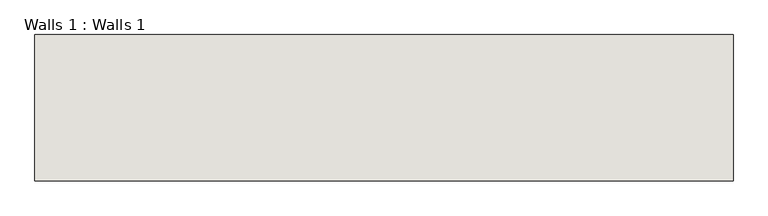
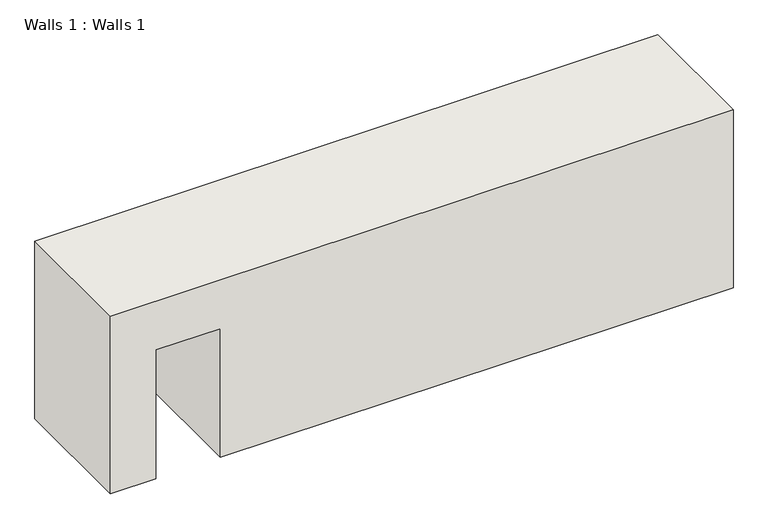
"""IFC4 building model written with IfcOpenShell, lengths in millimetres: wall geometry, Walls 1 : Walls 1."""

from ifc_helpers import new_model, si_unit, frame, origin, place, context, project, spatial, polyline, outline, extrude, source, transform, mapped, element, save


def walls_1_walls_1_b68e0aa0(model_context):
    return source(origin(), model_context, "Body", "SweptSolid", [
        extrude(outline(polyline([(3048.0, 11829.2591022), (3048.0, 1727.6505118), (0.0, 1727.6505118), (0.0, 2465.7505118), (2210.0, 2465.7505118), (2210.0, 3510.4263062), (0.0, 3510.4263062), (0.0, 11829.2591022), (3048.0, 11829.2591022)])), frame((0.0, -423.7652905, 0.0), z_axis=(0.0, 1.0, 0.0), x_axis=(0.0, 0.0, 1.0)), (0.0, 0.0, 1.0), 2119.4074841),
    ])


if __name__ == "__main__":
    model = new_model("IFC4")
    model_context = context("Model", 3, world=origin())
    ifc_project = project(units=[si_unit("LENGTHUNIT", "METRE", prefix="MILLI")], contexts=[model_context])
    site = spatial("IfcSite", under=ifc_project)
    building = spatial("IfcBuilding", under=site)
    placement = place(None, origin())
    walls_1_walls_1_shape = walls_1_walls_1_b68e0aa0(model_context)
    element("IfcWall", 1, ObjectType="Walls 1 : Walls 1", at=placement, inside=building, context=model_context, shape_type="MappedRepresentation", body=[
        mapped(walls_1_walls_1_shape, transform((0.0, 0.0, 0.0), x_axis=(1.0, 0.0, 0.0), y_axis=(0.0, 1.0, 0.0), z_axis=(0.0, 0.0, 1.0))),
    ])
    save(model, "model.ifc")

# Revit data of these elements
# Element 1 (IfcWall, "Walls 1 : Walls 1")
#   Materials on its faces: "Default Wall"
# Materials
#   "Default Wall": colour RGB 80 80 80, transparency 0
